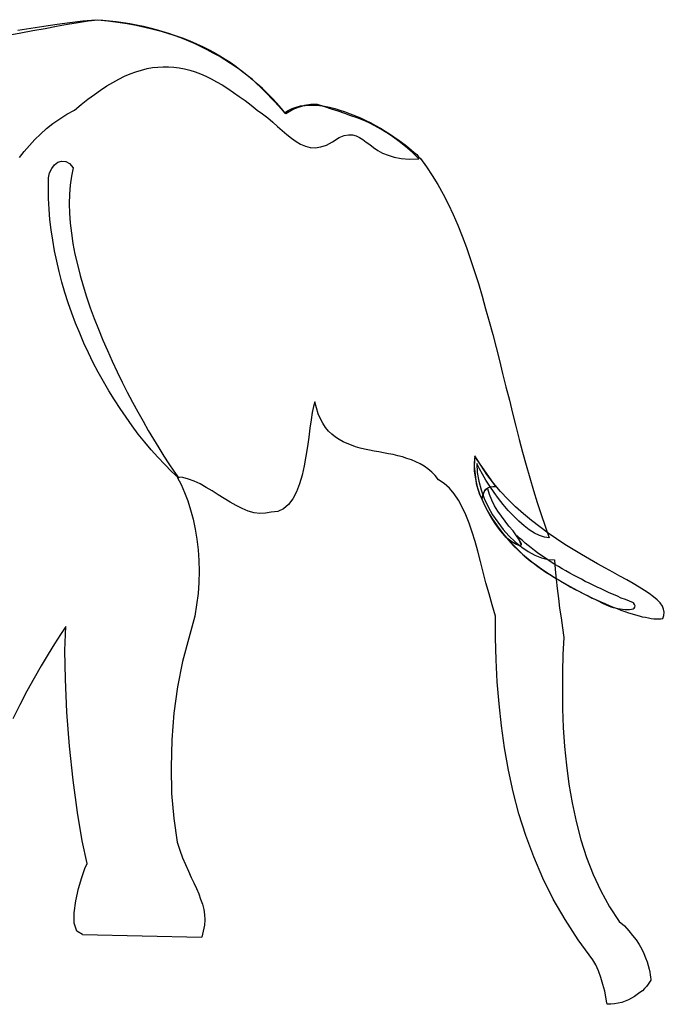
# Model space of a CAD drawing. Units: inches. Extents: x 386 to 107067, y -7 to 96314.
# Tile 10 of 10: x 107064.862 to 107066.855, y 96311.177 to 96314.222. Entities that reach past the tile are written whole.
import ezdxf

# ---------------------------------------------------------------- set-up
doc = ezdxf.new("R2010")
doc.units = ezdxf.units.IN
doc.layers.add('A-ELEV', color=7, linetype='Continuous', lineweight=25)
doc.layers.add('freecads.com', color=7, linetype='Continuous')

# ---------------------------------------------------------------- blocks, each defined once
blk = doc.blocks.new('elephant')
at = {"layer": 'freecads.com'}
for p, q in [((104458.6453, 95264.9047), (104458.6048, 95264.8987)), ((104458.6858, 95264.9107), (104458.6453, 95264.9047)), ((104458.6486, 95264.8987), (104458.6841, 95264.9052)), ((104458.6841, 95264.9052), (104458.7181, 95264.9113)), ((104458.7257, 95264.9162), (104458.6858, 95264.9107)), ((104458.7181, 95264.9113), (104458.7509, 95264.9167)), ((104458.7656, 95264.9206), (104458.7257, 95264.9162)), ((104458.7509, 95264.9167), (104458.782, 95264.9217)), ((104458.8055, 95264.9244), (104458.7656, 95264.9206)), ((104458.782, 95264.9217), (104458.8116, 95264.9255)), ((104458.8269, 95264.9227), (104458.8055, 95264.9244)), ((104458.8116, 95264.9255), (104458.8427, 95264.9222)), ((104458.8482, 95264.9211), (104458.8269, 95264.9227)), ((104458.8427, 95264.9222), (104458.8734, 95264.9178)), ((104458.869, 95264.9189), (104458.8482, 95264.9211)), ((104458.8903, 95264.9156), (104458.869, 95264.9189)), ((104458.8734, 95264.9178), (104458.9023, 95264.9134)), ((104458.9111, 95264.9124), (104458.8903, 95264.9156)), ((104458.9023, 95264.9134), (104458.9302, 95264.9085)), ((104458.9319, 95264.9085), (104458.9111, 95264.9124)), ((104458.9302, 95264.9085), (104458.957, 95264.9025)), ((104458.9527, 95264.9041), (104458.9319, 95264.9085)), ((104458.9734, 95264.8992), (104458.9527, 95264.9041)), ((104458.957, 95264.9025), (104458.9827, 95264.8965)), ((104458.5348, 95264.8773), (104458.5737, 95264.885)), ((104458.6048, 95264.8987), (104458.5644, 95264.8921)), ((104458.5737, 95264.885), (104458.6114, 95264.8921)), ((104458.6114, 95264.8921), (104458.6486, 95264.8987)), ((104458.9937, 95264.8938), (104458.9734, 95264.8992)), ((104458.9827, 95264.8965), (104459.0073, 95264.8899)), ((104459.0139, 95264.8877), (104458.9937, 95264.8938)), ((104459.0073, 95264.8899), (104459.0308, 95264.8828)), ((104459.0341, 95264.8812), (104459.0139, 95264.8877)), ((104459.0308, 95264.8828), (104459.0538, 95264.8757)), ((104459.0538, 95264.8741), (104459.0341, 95264.8812)), ((104459.0538, 95264.8757), (104459.0757, 95264.8681)), ((104459.0735, 95264.867), (104459.0538, 95264.8741)), ((104459.0932, 95264.8588), (104459.0735, 95264.867)), ((104459.0757, 95264.8681), (104459.0965, 95264.8599)), ((104459.1123, 95264.8506), (104459.0932, 95264.8588)), ((104459.0965, 95264.8599), (104459.1167, 95264.8511)), ((104459.1315, 95264.8418), (104459.1123, 95264.8506)), ((104459.1167, 95264.8511), (104459.1359, 95264.8424)), ((104459.1501, 95264.832), (104459.1315, 95264.8418)), ((104459.1359, 95264.8424), (104459.1544, 95264.8331)), ((104459.1687, 95264.8221), (104459.1501, 95264.832)), ((104459.1544, 95264.8331), (104459.1719, 95264.8238)), ((104459.1867, 95264.8123), (104459.1687, 95264.8221)), ((104459.1719, 95264.8238), (104459.1889, 95264.8139)), ((104459.2048, 95264.8013), (104459.1867, 95264.8123)), ((104459.1889, 95264.8139), (104459.2053, 95264.8035)), ((104458.9811, 95264.7773), (104458.9975, 95264.7789)), ((104458.9975, 95264.7789), (104459.0139, 95264.78)), ((104459.0139, 95264.78), (104459.0303, 95264.78)), ((104459.0303, 95264.78), (104459.0467, 95264.7789)), ((104459.0467, 95264.7789), (104459.0631, 95264.7767)), ((104459.2223, 95264.7899), (104459.2048, 95264.8013)), ((104459.2053, 95264.8035), (104459.2212, 95264.7937)), ((104459.2212, 95264.7937), (104459.2359, 95264.7833)), ((104459.2398, 95264.7784), (104459.2223, 95264.7899)), ((104459.2359, 95264.7833), (104459.2502, 95264.7724)), ((104458.8766, 95264.7412), (104458.8947, 95264.7505)), ((104458.8947, 95264.7505), (104458.9122, 95264.7581)), ((104458.9122, 95264.7581), (104458.9297, 95264.7642)), ((104458.9297, 95264.7642), (104458.9472, 95264.7696)), ((104458.9472, 95264.7696), (104458.9641, 95264.774)), ((104458.9641, 95264.774), (104458.9811, 95264.7773)), ((104459.0631, 95264.7767), (104459.0795, 95264.7735)), ((104459.0795, 95264.7735), (104459.0959, 95264.7691)), ((104459.0959, 95264.7691), (104459.1123, 95264.7642)), ((104459.1123, 95264.7642), (104459.1288, 95264.7576)), ((104459.1288, 95264.7576), (104459.1457, 95264.7505)), ((104459.1457, 95264.7505), (104459.1621, 95264.7423)), ((104459.2567, 95264.7658), (104459.2398, 95264.7784)), ((104459.2502, 95264.7724), (104459.2644, 95264.7614)), ((104459.2737, 95264.7532), (104459.2567, 95264.7658)), ((104459.2644, 95264.7614), (104459.2775, 95264.7505)), ((104459.2901, 95264.7401), (104459.2737, 95264.7532)), ((104459.2775, 95264.7505), (104459.2906, 95264.7395)), ((104458.8203, 95264.7078), (104458.8395, 95264.7204)), ((104458.8395, 95264.7204), (104458.8581, 95264.7313)), ((104458.8581, 95264.7313), (104458.8766, 95264.7412)), ((104459.1621, 95264.7423), (104459.179, 95264.7335)), ((104459.179, 95264.7335), (104459.196, 95264.7237)), ((104459.196, 95264.7237), (104459.2135, 95264.7128)), ((104459.3059, 95264.7264), (104459.2901, 95264.7401)), ((104459.2906, 95264.7395), (104459.3026, 95264.7281)), ((104459.3026, 95264.7281), (104459.3147, 95264.7171)), ((104459.3212, 95264.7122), (104459.3059, 95264.7264)), ((104458.7809, 95264.6794), (104458.8012, 95264.6942)), ((104458.8012, 95264.6942), (104458.8203, 95264.7078)), ((104459.2135, 95264.7128), (104459.231, 95264.7007)), ((104459.231, 95264.7007), (104459.2491, 95264.6882)), ((104459.2491, 95264.6882), (104459.2671, 95264.675)), ((104459.3147, 95264.7171), (104459.3262, 95264.7056)), ((104459.3366, 95264.6974), (104459.3212, 95264.7122)), ((104459.3262, 95264.7056), (104459.3376, 95264.6942)), ((104459.3513, 95264.6827), (104459.3366, 95264.6974)), ((104459.3376, 95264.6942), (104459.348, 95264.6827)), ((104458.7399, 95264.6455), (104458.7607, 95264.663)), ((104458.7607, 95264.663), (104458.7809, 95264.6794)), ((104459.2671, 95264.675), (104459.2857, 95264.6608)), ((104459.2857, 95264.6608), (104459.3043, 95264.6455)), ((104459.348, 95264.6827), (104459.359, 95264.6712)), ((104459.3655, 95264.6668), (104459.3513, 95264.6827)), ((104459.359, 95264.6712), (104459.3694, 95264.6597)), ((104459.3792, 95264.651), (104459.3655, 95264.6668)), ((104459.3694, 95264.6597), (104459.3792, 95264.6488)), ((104459.4251, 95264.6553), (104459.4383, 95264.6586)), ((104459.4383, 95264.6586), (104459.4525, 95264.6603)), ((104459.4443, 95264.6581), (104459.4383, 95264.6564)), ((104459.4508, 95264.6597), (104459.4443, 95264.6581)), ((104459.4574, 95264.6613), (104459.4508, 95264.6597)), ((104459.4525, 95264.6603), (104459.4667, 95264.6613)), ((104459.464, 95264.6624), (104459.4574, 95264.6613)), ((104459.4705, 95264.663), (104459.464, 95264.6624)), ((104459.4667, 95264.6613), (104459.4815, 95264.6613)), ((104459.4771, 95264.6635), (104459.4705, 95264.663)), ((104459.4842, 95264.6635), (104459.4771, 95264.6635)), ((104459.4815, 95264.6613), (104459.4968, 95264.6603)), ((104459.4908, 95264.663), (104459.4842, 95264.6635)), ((104459.5132, 95264.6559), (104459.4908, 95264.663)), ((104459.4968, 95264.6603), (104459.5127, 95264.6581)), ((104459.5127, 95264.6581), (104459.528, 95264.6548)), ((104458.6945, 95264.6192), (104458.7164, 95264.6329)), ((104458.7164, 95264.6329), (104458.7399, 95264.6455)), ((104459.3043, 95264.6455), (104459.3212, 95264.634)), ((104459.3212, 95264.634), (104459.3371, 95264.6214)), ((104459.3929, 95264.6345), (104459.3792, 95264.651)), ((104459.3792, 95264.6488), (104459.3891, 95264.6373)), ((104459.3891, 95264.6373), (104459.4005, 95264.6444)), ((104459.3978, 95264.6378), (104459.3929, 95264.6345)), ((104459.4033, 95264.6406), (104459.3978, 95264.6378)), ((104459.4005, 95264.6444), (104459.4126, 95264.6504)), ((104459.4087, 95264.6433), (104459.4033, 95264.6406)), ((104459.4142, 95264.6466), (104459.4087, 95264.6433)), ((104459.4126, 95264.6504), (104459.4251, 95264.6553)), ((104459.4197, 95264.6493), (104459.4142, 95264.6466)), ((104459.4257, 95264.6515), (104459.4197, 95264.6493)), ((104459.4317, 95264.6542), (104459.4257, 95264.6515)), ((104459.4383, 95264.6564), (104459.4317, 95264.6542)), ((104459.5345, 95264.6488), (104459.5132, 95264.6559)), ((104459.528, 95264.6548), (104459.5444, 95264.651)), ((104459.5553, 95264.6422), (104459.5345, 95264.6488)), ((104459.5444, 95264.651), (104459.5602, 95264.646)), ((104459.575, 95264.6356), (104459.5553, 95264.6422)), ((104459.5602, 95264.646), (104459.5761, 95264.6406)), ((104459.5941, 95264.6285), (104459.575, 95264.6356)), ((104459.5761, 95264.6406), (104459.5925, 95264.6345)), ((104459.5925, 95264.6345), (104459.6083, 95264.6285)), ((104459.6133, 95264.622), (104459.5941, 95264.6285)), ((104459.6083, 95264.6285), (104459.6242, 95264.6214)), ((104458.6535, 95264.5886), (104458.6732, 95264.6045)), ((104458.6732, 95264.6045), (104458.6945, 95264.6192)), ((104459.3371, 95264.6214), (104459.353, 95264.6083)), ((104459.353, 95264.6083), (104459.3677, 95264.5952)), ((104459.6319, 95264.6143), (104459.6133, 95264.622)), ((104459.6242, 95264.6214), (104459.6401, 95264.6138)), ((104459.6505, 95264.6061), (104459.6319, 95264.6143)), ((104459.6401, 95264.6138), (104459.6554, 95264.6061)), ((104459.6685, 95264.5974), (104459.6505, 95264.6061)), ((104459.6554, 95264.6061), (104459.6707, 95264.5979)), ((104459.6865, 95264.587), (104459.6685, 95264.5974)), ((104459.6707, 95264.5979), (104459.6855, 95264.5897)), ((104458.6174, 95264.5547), (104458.6349, 95264.5717)), ((104458.6349, 95264.5717), (104458.6535, 95264.5886)), ((104459.3677, 95264.5952), (104459.382, 95264.5826)), ((104459.382, 95264.5826), (104459.3962, 95264.57)), ((104459.3962, 95264.57), (104459.4104, 95264.5585)), ((104459.5575, 95264.5613), (104459.5733, 95264.5673)), ((104459.5733, 95264.5673), (104459.587, 95264.5695)), ((104459.587, 95264.5695), (104459.5996, 95264.5689)), ((104459.5996, 95264.5689), (104459.6105, 95264.5662)), ((104459.6105, 95264.5662), (104459.6209, 95264.5613)), ((104459.6855, 95264.5897), (104459.6997, 95264.581)), ((104459.7051, 95264.576), (104459.6865, 95264.587)), ((104459.6997, 95264.581), (104459.7133, 95264.5722)), ((104459.7243, 95264.5629), (104459.7051, 95264.576)), ((104459.7133, 95264.5722), (104459.7265, 95264.5635)), ((104458.5846, 95264.5181), (104458.6005, 95264.5367)), ((104458.6005, 95264.5367), (104458.6174, 95264.5547)), ((104459.4104, 95264.5585), (104459.4246, 95264.5487)), ((104459.4246, 95264.5487), (104459.4388, 95264.5405)), ((104459.4388, 95264.5405), (104459.4536, 95264.5345)), ((104459.5012, 95264.5317), (104459.5187, 95264.5378)), ((104459.5187, 95264.5378), (104459.5373, 95264.5476)), ((104459.5373, 95264.5476), (104459.5575, 95264.5613)), ((104459.6209, 95264.5613), (104459.6313, 95264.5547)), ((104459.6313, 95264.5547), (104459.6417, 95264.5471)), ((104459.6417, 95264.5471), (104459.6526, 95264.5389)), ((104459.6526, 95264.5389), (104459.6641, 95264.5301)), ((104459.7434, 95264.5487), (104459.7243, 95264.5629)), ((104459.7265, 95264.5635), (104459.739, 95264.5553)), ((104459.739, 95264.5553), (104459.7511, 95264.5465)), ((104459.7631, 95264.5328), (104459.7434, 95264.5487)), ((104459.7511, 95264.5465), (104459.762, 95264.5383)), ((104459.762, 95264.5383), (104459.7724, 95264.5301)), ((104458.5693, 95264.4995), (104458.5846, 95264.5181)), ((104459.4536, 95264.5345), (104459.4683, 95264.5306)), ((104459.4683, 95264.5306), (104459.4842, 95264.5296)), ((104459.4842, 95264.5296), (104459.5012, 95264.5317)), ((104459.6641, 95264.5301), (104459.6773, 95264.5213)), ((104459.6773, 95264.5213), (104459.692, 95264.5131)), ((104459.692, 95264.5131), (104459.709, 95264.506)), ((104459.709, 95264.506), (104459.7281, 95264.5)), ((104459.7833, 95264.5153), (104459.7631, 95264.5328)), ((104459.7724, 95264.5301), (104459.7817, 95264.5224)), ((104459.7817, 95264.5224), (104459.7899, 95264.5148)), ((104459.8047, 95264.4951), (104459.7833, 95264.5153)), ((104459.7899, 95264.5148), (104459.7976, 95264.5082)), ((104459.7976, 95264.5082), (104459.8036, 95264.5017)), ((104458.6694, 95264.4656), (104458.6781, 95264.4765)), ((104458.6781, 95264.4765), (104458.6885, 95264.4847)), ((104458.6885, 95264.4847), (104458.7, 95264.488)), ((104458.7, 95264.488), (104458.7126, 95264.4869)), ((104458.7126, 95264.4869), (104458.7246, 95264.4803)), ((104458.7246, 95264.4803), (104458.7361, 95264.4672)), ((104459.7281, 95264.5), (104459.75, 95264.4962)), ((104459.75, 95264.4962), (104459.7757, 95264.4945)), ((104459.7757, 95264.4945), (104459.8047, 95264.4951)), ((104459.8036, 95264.5017), (104459.809, 95264.4956)), ((104459.809, 95264.4956), (104459.8276, 95264.4705)), ((104458.6595, 95264.436), (104458.6628, 95264.4519)), ((104458.6628, 95264.4519), (104458.6694, 95264.4656)), ((104458.7361, 95264.4672), (104458.7301, 95264.441)), ((104459.8276, 95264.4705), (104459.8457, 95264.4437)), ((104459.8457, 95264.4437), (104459.8632, 95264.4158)), ((104458.659, 95264.4043), (104458.6595, 95264.436)), ((104458.7263, 95264.4136), (104458.7241, 95264.3857)), ((104458.7301, 95264.441), (104458.7263, 95264.4136)), ((104459.8632, 95264.4158), (104459.8796, 95264.3863)), ((104458.6595, 95264.3721), (104458.659, 95264.4043)), ((104458.7241, 95264.3857), (104458.723, 95264.3562)), ((104459.8796, 95264.3863), (104459.8949, 95264.3556)), ((104458.6612, 95264.3398), (104458.6595, 95264.3721)), ((104458.723, 95264.3562), (104458.7241, 95264.3267)), ((104459.8949, 95264.3556), (104459.9102, 95264.3234)), ((104458.6639, 95264.3075), (104458.6612, 95264.3398)), ((104458.7241, 95264.3267), (104458.7263, 95264.296)), ((104459.9102, 95264.3234), (104459.9244, 95264.29)), ((104458.6677, 95264.2753), (104458.6639, 95264.3075)), ((104458.7263, 95264.296), (104458.7301, 95264.2649)), ((104458.6727, 95264.243), (104458.6677, 95264.2753)), ((104458.7301, 95264.2649), (104458.735, 95264.2331)), ((104459.9244, 95264.29), (104459.9381, 95264.2556)), ((104458.6781, 95264.2107), (104458.6727, 95264.243)), ((104458.735, 95264.2331), (104458.741, 95264.2003)), ((104459.9381, 95264.2556), (104459.9512, 95264.2206)), ((104458.6847, 95264.1785), (104458.6781, 95264.2107)), ((104458.741, 95264.2003), (104458.7487, 95264.1681)), ((104459.9512, 95264.2206), (104459.9643, 95264.1839)), ((104458.6924, 95264.1462), (104458.6847, 95264.1785)), ((104459.9643, 95264.1839), (104459.9764, 95264.1468)), ((104458.7011, 95264.1139), (104458.6924, 95264.1462)), ((104458.7487, 95264.1681), (104458.7569, 95264.1347)), ((104459.9764, 95264.1468), (104459.9884, 95264.109)), ((104458.7104, 95264.0817), (104458.7011, 95264.1139)), ((104458.7569, 95264.1347), (104458.7667, 95264.1019)), ((104459.9884, 95264.109), (104459.9999, 95264.0707)), ((104458.7202, 95264.0499), (104458.7104, 95264.0817)), ((104458.7667, 95264.1019), (104458.7771, 95264.0685)), ((104458.7312, 95264.0182), (104458.7202, 95264.0499)), ((104458.7771, 95264.0685), (104458.7886, 95264.0346)), ((104459.9999, 95264.0707), (104460.0108, 95264.0314)), ((104458.7432, 95263.9871), (104458.7312, 95264.0182)), ((104458.7886, 95264.0346), (104458.8006, 95264.0013)), ((104460.0108, 95264.0314), (104460.0218, 95263.992)), ((104458.7558, 95263.9559), (104458.7432, 95263.9871)), ((104458.8006, 95264.0013), (104458.8138, 95263.9679)), ((104460.0218, 95263.992), (104460.0327, 95263.9521)), ((104458.8138, 95263.9679), (104458.8274, 95263.9346)), ((104458.7689, 95263.9253), (104458.7558, 95263.9559)), ((104458.8274, 95263.9346), (104458.8416, 95263.9018)), ((104460.0327, 95263.9521), (104460.0431, 95263.9116)), ((104458.7831, 95263.8946), (104458.7689, 95263.9253)), ((104458.8416, 95263.9018), (104458.8559, 95263.8689)), ((104460.0431, 95263.9116), (104460.0535, 95263.8711)), ((104458.7973, 95263.8646), (104458.7831, 95263.8946)), ((104458.8559, 95263.8689), (104458.8712, 95263.8367)), ((104460.0535, 95263.8711), (104460.0633, 95263.8307)), ((104458.8132, 95263.835), (104458.7973, 95263.8646)), ((104458.8291, 95263.806), (104458.8132, 95263.835)), ((104458.8712, 95263.8367), (104458.887, 95263.8044)), ((104458.8455, 95263.7776), (104458.8291, 95263.806)), ((104458.887, 95263.8044), (104458.9029, 95263.7732)), ((104460.0633, 95263.8307), (104460.0737, 95263.7896)), ((104458.863, 95263.7497), (104458.8455, 95263.7776)), ((104460.0737, 95263.7896), (104460.0841, 95263.7486)), ((104458.8805, 95263.7224), (104458.863, 95263.7497)), ((104458.9029, 95263.7732), (104458.9187, 95263.7426)), ((104459.4831, 95263.7437), (104459.4787, 95263.7289)), ((104459.4875, 95263.7246), (104459.4831, 95263.7437)), ((104460.0841, 95263.7486), (104460.094, 95263.7082)), ((104458.8991, 95263.6956), (104458.8805, 95263.7224)), ((104458.9187, 95263.7426), (104458.9352, 95263.7125)), ((104459.4787, 95263.7289), (104459.4749, 95263.7103)), ((104459.4935, 95263.7065), (104459.4875, 95263.7246)), ((104458.9176, 95263.6694), (104458.8991, 95263.6956)), ((104458.9352, 95263.7125), (104458.9516, 95263.6835)), ((104458.9516, 95263.6835), (104458.968, 95263.6551)), ((104459.4711, 95263.6874), (104459.4678, 95263.6622)), ((104459.4749, 95263.7103), (104459.4711, 95263.6874)), ((104459.5001, 95263.6912), (104459.4935, 95263.7065)), ((104459.5077, 95263.677), (104459.5001, 95263.6912)), ((104460.094, 95263.7082), (104460.1043, 95263.6677)), ((104458.9368, 95263.6436), (104458.9176, 95263.6694)), ((104458.968, 95263.6551), (104458.9838, 95263.6278)), ((104459.4678, 95263.6622), (104459.464, 95263.6343)), ((104459.5159, 95263.6639), (104459.5077, 95263.677)), ((104459.5252, 95263.6529), (104459.5159, 95263.6639)), ((104459.5356, 95263.6431), (104459.5252, 95263.6529)), ((104460.1043, 95263.6677), (104460.1147, 95263.6272)), ((104458.957, 95263.619), (104458.9368, 95263.6436)), ((104458.9838, 95263.6278), (104459.0002, 95263.601)), ((104459.464, 95263.6343), (104459.4601, 95263.6054)), ((104459.5466, 95263.6343), (104459.5356, 95263.6431)), ((104459.558, 95263.6267), (104459.5466, 95263.6343)), ((104459.5701, 95263.6196), (104459.558, 95263.6267)), ((104460.1147, 95263.6272), (104460.1251, 95263.5873)), ((104458.9773, 95263.595), (104458.957, 95263.619)), ((104458.9975, 95263.572), (104458.9773, 95263.595)), ((104459.0002, 95263.601), (104459.0161, 95263.5758)), ((104459.4601, 95263.6054), (104459.4552, 95263.5753)), ((104459.5826, 95263.6141), (104459.5701, 95263.6196)), ((104459.5958, 95263.6092), (104459.5826, 95263.6141)), ((104459.6089, 95263.6043), (104459.5958, 95263.6092)), ((104459.6226, 95263.6004), (104459.6089, 95263.6043)), ((104459.6368, 95263.5972), (104459.6226, 95263.6004)), ((104459.6516, 95263.5944), (104459.6368, 95263.5972)), ((104459.6658, 95263.5912), (104459.6516, 95263.5944)), ((104459.6805, 95263.5884), (104459.6658, 95263.5912)), ((104459.0188, 95263.5496), (104458.9975, 95263.572)), ((104459.0161, 95263.5758), (104459.0319, 95263.5518)), ((104459.4552, 95263.5753), (104459.4497, 95263.5458)), ((104459.6953, 95263.5857), (104459.6805, 95263.5884)), ((104459.7101, 95263.583), (104459.6953, 95263.5857)), ((104459.7248, 95263.5802), (104459.7101, 95263.583)), ((104459.739, 95263.5769), (104459.7248, 95263.5802)), ((104459.7533, 95263.5731), (104459.739, 95263.5769)), ((104459.7675, 95263.5687), (104459.7533, 95263.5731)), ((104459.7817, 95263.5638), (104459.7675, 95263.5687)), ((104459.7948, 95263.5583), (104459.7817, 95263.5638)), ((104459.9775, 95263.5769), (104459.9753, 95263.5534)), ((104459.9764, 95263.5605), (104459.9758, 95263.5447)), ((104459.9775, 95263.5748), (104459.9764, 95263.5605)), ((104459.9955, 95263.5474), (104459.9775, 95263.5769)), ((104460.042, 95263.4812), (104459.9775, 95263.5748)), ((104460.1251, 95263.5873), (104460.1361, 95263.5474)), ((104459.0401, 95263.5283), (104459.0188, 95263.5496)), ((104459.0319, 95263.5518), (104459.0473, 95263.5288)), ((104459.4497, 95263.5458), (104459.4432, 95263.5168)), ((104459.808, 95263.5518), (104459.7948, 95263.5583)), ((104459.8205, 95263.5441), (104459.808, 95263.5518)), ((104459.8326, 95263.5359), (104459.8205, 95263.5441)), ((104459.8446, 95263.5261), (104459.8326, 95263.5359)), ((104459.9753, 95263.5534), (104459.9758, 95263.5294)), ((104459.9758, 95263.5447), (104459.9769, 95263.5272)), ((104459.9917, 95263.5365), (104459.9835, 95263.5523)), ((104459.9835, 95263.5523), (104459.9851, 95263.525)), ((104460.001, 95263.5195), (104459.9917, 95263.5365)), ((104460.0147, 95263.519), (104459.9955, 95263.5474)), ((104460.1361, 95263.5474), (104460.147, 95263.5086)), ((104459.062, 95263.5075), (104459.0401, 95263.5283)), ((104459.0473, 95263.5288), (104459.062, 95263.5075)), ((104459.0746, 95263.5091), (104459.0576, 95263.5108)), ((104459.0576, 95263.5108), (104459.0691, 95263.4878)), ((104459.0921, 95263.5047), (104459.0746, 95263.5091)), ((104459.1102, 95263.4982), (104459.0921, 95263.5047)), ((104459.4432, 95263.5168), (104459.4355, 95263.49)), ((104459.855, 95263.5151), (104459.8446, 95263.5261)), ((104459.8654, 95263.5026), (104459.855, 95263.5151)), ((104459.8829, 95263.4911), (104459.8654, 95263.5026)), ((104459.9758, 95263.5294), (104459.9791, 95263.5053)), ((104459.9769, 95263.5272), (104459.9791, 95263.5091)), ((104459.9791, 95263.5091), (104459.9818, 95263.4911)), ((104459.9791, 95263.5053), (104459.9851, 95263.4807)), ((104459.9851, 95263.525), (104459.9895, 95263.4976)), ((104460.0119, 95263.5009), (104460.001, 95263.5195)), ((104460.024, 95263.4823), (104460.0119, 95263.5009)), ((104460.0349, 95263.4922), (104460.0147, 95263.519)), ((104460.147, 95263.5086), (104460.1585, 95263.4697)), ((104459.0691, 95263.4878), (104459.0801, 95263.4632)), ((104459.1282, 95263.4894), (104459.1102, 95263.4982)), ((104459.1468, 95263.479), (104459.1282, 95263.4894)), ((104459.1654, 95263.4681), (104459.1468, 95263.479)), ((104459.4355, 95263.49), (104459.4257, 95263.4648)), ((104459.8987, 95263.4763), (104459.8829, 95263.4911)), ((104459.9135, 95263.4594), (104459.8987, 95263.4763)), ((104459.9818, 95263.4911), (104459.9868, 95263.4736)), ((104459.9851, 95263.4807), (104459.9933, 95263.4561)), ((104459.9868, 95263.4736), (104459.9922, 95263.4572)), ((104459.9895, 95263.4976), (104459.9966, 95263.4708)), ((104459.9966, 95263.4708), (104460.0065, 95263.4446)), ((104460.007, 95263.4676), (104460.0119, 95263.4736)), ((104460.0103, 95263.4703), (104460.0076, 95263.467)), ((104460.0136, 95263.473), (104460.0103, 95263.4703)), ((104460.0119, 95263.4736), (104460.0179, 95263.4774)), ((104460.0174, 95263.4747), (104460.0136, 95263.473)), ((104460.0229, 95263.4566), (104460.0174, 95263.4747)), ((104460.0179, 95263.4774), (104460.0245, 95263.4801)), ((104460.0371, 95263.4632), (104460.024, 95263.4823)), ((104460.0245, 95263.4801), (104460.0327, 95263.4812)), ((104460.0327, 95263.4812), (104460.042, 95263.4812)), ((104460.0568, 95263.4665), (104460.0349, 95263.4922)), ((104460.1585, 95263.4697), (104460.17, 95263.432)), ((104459.0801, 95263.4632), (104459.0899, 95263.4369)), ((104459.184, 95263.4561), (104459.1654, 95263.4681)), ((104459.2026, 95263.4446), (104459.184, 95263.4561)), ((104459.2212, 95263.4331), (104459.2026, 95263.4446)), ((104459.4148, 95263.4435), (104459.4016, 95263.4255)), ((104459.4257, 95263.4648), (104459.4148, 95263.4435)), ((104459.9266, 95263.4397), (104459.9135, 95263.4594)), ((104459.9387, 95263.4178), (104459.9266, 95263.4397)), ((104459.9922, 95263.4572), (104459.9999, 95263.4424)), ((104459.9933, 95263.4561), (104460.0037, 95263.4315)), ((104460.0004, 95263.4473), (104459.9988, 95263.4419)), ((104459.9988, 95263.4419), (104460.0065, 95263.4255)), ((104459.9999, 95263.4424), (104460.001, 95263.4522)), ((104460.0021, 95263.4528), (104460.0004, 95263.4473)), ((104460.001, 95263.4522), (104460.0037, 95263.461)), ((104460.0032, 95263.4577), (104460.0021, 95263.4528)), ((104460.0054, 95263.4626), (104460.0032, 95263.4577)), ((104460.0037, 95263.461), (104460.007, 95263.4676)), ((104460.0076, 95263.467), (104460.0054, 95263.4626)), ((104460.0065, 95263.4446), (104460.0185, 95263.4189)), ((104460.03, 95263.4397), (104460.0229, 95263.4566)), ((104460.0387, 95263.4222), (104460.03, 95263.4397)), ((104460.0508, 95263.444), (104460.0371, 95263.4632)), ((104460.0655, 95263.4255), (104460.0508, 95263.444)), ((104460.0797, 95263.4424), (104460.0568, 95263.4665)), ((104460.1033, 95263.4189), (104460.0797, 95263.4424)), ((104459.0899, 95263.4369), (104459.0987, 95263.4091)), ((104459.0987, 95263.4091), (104459.1063, 95263.3801)), ((104459.2398, 95263.4227), (104459.2212, 95263.4331)), ((104459.2584, 95263.4134), (104459.2398, 95263.4227)), ((104459.2769, 95263.4058), (104459.2584, 95263.4134)), ((104459.3858, 95263.4123), (104459.3683, 95263.4041)), ((104459.4016, 95263.4255), (104459.3858, 95263.4123)), ((104459.9496, 95263.3937), (104459.9387, 95263.4178)), ((104460.0037, 95263.4315), (104460.0158, 95263.4074)), ((104460.0065, 95263.4255), (104460.0141, 95263.4101)), ((104460.0141, 95263.4101), (104460.0212, 95263.3965)), ((104460.0185, 95263.4189), (104460.0322, 95263.3943)), ((104460.0486, 95263.4058), (104460.0387, 95263.4222)), ((104460.0808, 95263.4074), (104460.0655, 95263.4255)), ((104460.1279, 95263.397), (104460.1033, 95263.4189)), ((104460.17, 95263.432), (104460.182, 95263.3948)), ((104459.1063, 95263.3801), (104459.1129, 95263.3494)), ((104459.295, 95263.4003), (104459.2769, 95263.4058)), ((104459.313, 95263.3981), (104459.295, 95263.4003)), ((104459.3305, 95263.3987), (104459.313, 95263.3981)), ((104459.3475, 95263.4025), (104459.3305, 95263.3987)), ((104459.3683, 95263.4041), (104459.3475, 95263.4025)), ((104459.9594, 95263.368), (104459.9496, 95263.3937)), ((104460.0158, 95263.4074), (104460.03, 95263.3833)), ((104460.0212, 95263.3965), (104460.0289, 95263.3833)), ((104460.0289, 95263.3833), (104460.0371, 95263.3702)), ((104460.03, 95263.3833), (104460.0464, 95263.3598)), ((104460.0322, 95263.3943), (104460.048, 95263.3708)), ((104460.0595, 95263.3899), (104460.0486, 95263.4058)), ((104460.071, 95263.374), (104460.0595, 95263.3899)), ((104460.0967, 95263.3905), (104460.0808, 95263.4074)), ((104460.1131, 95263.3746), (104460.0967, 95263.3905)), ((104460.1525, 95263.3762), (104460.1279, 95263.397)), ((104460.182, 95263.3948), (104460.1946, 95263.3587)), ((104459.1129, 95263.3494), (104459.1178, 95263.3183)), ((104459.9687, 95263.3407), (104459.9594, 95263.368)), ((104460.0371, 95263.3702), (104460.0464, 95263.3571)), ((104460.0464, 95263.3598), (104460.0639, 95263.3363)), ((104460.0464, 95263.3571), (104460.0568, 95263.3434)), ((104460.048, 95263.3708), (104460.065, 95263.3489)), ((104460.065, 95263.3489), (104460.083, 95263.3287)), ((104460.083, 95263.3587), (104460.071, 95263.374)), ((104460.0956, 95263.344), (104460.083, 95263.3587)), ((104460.1295, 95263.3598), (104460.1131, 95263.3746)), ((104460.1454, 95263.3478), (104460.1295, 95263.3598)), ((104460.1618, 95263.3374), (104460.1454, 95263.3478)), ((104460.1782, 95263.3565), (104460.1525, 95263.3762)), ((104460.2039, 95263.3374), (104460.1782, 95263.3565)), ((104460.1946, 95263.3587), (104460.2077, 95263.3232)), ((104459.1178, 95263.3183), (104459.1216, 95263.286)), ((104459.978, 95263.3117), (104459.9687, 95263.3407)), ((104460.0568, 95263.3434), (104460.0688, 95263.3287)), ((104460.0639, 95263.3363), (104460.083, 95263.3144)), ((104460.0688, 95263.3287), (104460.0715, 95263.3265)), ((104460.0715, 95263.3265), (104460.0754, 95263.3237)), ((104460.0754, 95263.3237), (104460.0803, 95263.3199)), ((104460.0803, 95263.3199), (104460.0863, 95263.3155)), ((104460.083, 95263.3287), (104460.1022, 95263.3101)), ((104460.106, 95263.3292), (104460.0956, 95263.344)), ((104460.1136, 95263.3183), (104460.106, 95263.3292)), ((104460.1076, 95263.3297), (104460.1125, 95263.321)), ((104460.1158, 95263.3221), (104460.1076, 95263.3297)), ((104460.1125, 95263.321), (104460.1169, 95263.3128)), ((104460.118, 95263.3095), (104460.1136, 95263.3183)), ((104460.1246, 95263.3144), (104460.1158, 95263.3221)), ((104460.1776, 95263.3297), (104460.1618, 95263.3374)), ((104460.193, 95263.3248), (104460.1776, 95263.3297)), ((104460.2077, 95263.3232), (104460.193, 95263.3248)), ((104460.2301, 95263.3194), (104460.2039, 95263.3374)), ((104460.2558, 95263.3024), (104460.2301, 95263.3194)), ((104459.9862, 95263.2811), (104459.978, 95263.3117)), ((104460.1, 95263.3051), (104460.0814, 95263.3161)), ((104460.0814, 95263.3161), (104460.0961, 95263.2991)), ((104460.083, 95263.3144), (104460.1038, 95263.2926)), ((104460.0863, 95263.3155), (104460.0923, 95263.3112)), ((104460.0923, 95263.3112), (104460.0989, 95263.3073)), ((104460.0961, 95263.2991), (104460.1125, 95263.2833)), ((104460.0989, 95263.3073), (104460.1049, 95263.3035)), ((104460.112, 95263.2997), (104460.1, 95263.3051)), ((104460.1022, 95263.3101), (104460.1224, 95263.2942)), ((104460.1038, 95263.2926), (104460.1251, 95263.2718)), ((104460.1049, 95263.3035), (104460.1104, 95263.3008)), ((104460.1104, 95263.3008), (104460.1147, 95263.2991)), ((104460.1186, 95263.2986), (104460.112, 95263.2997)), ((104460.1147, 95263.2991), (104460.1186, 95263.2991)), ((104460.1169, 95263.3128), (104460.1202, 95263.3057)), ((104460.1202, 95263.3041), (104460.118, 95263.3095)), ((104460.1207, 95263.3008), (104460.1186, 95263.2986)), ((104460.1186, 95263.2991), (104460.1202, 95263.3002)), ((104460.1202, 95263.3057), (104460.1207, 95263.3008)), ((104460.1202, 95263.3002), (104460.1202, 95263.3041)), ((104460.1224, 95263.2942), (104460.1426, 95263.2805)), ((104460.1333, 95263.3068), (104460.1246, 95263.3144)), ((104460.1426, 95263.2991), (104460.1333, 95263.3068)), ((104460.1519, 95263.2915), (104460.1426, 95263.2991)), ((104460.1618, 95263.2838), (104460.1519, 95263.2915)), ((104460.2815, 95263.2866), (104460.2558, 95263.3024)), ((104460.3072, 95263.2712), (104460.2815, 95263.2866)), ((104459.1216, 95263.286), (104459.1238, 95263.2532)), ((104459.995, 95263.2499), (104459.9862, 95263.2811)), ((104460.1125, 95263.2833), (104460.13, 95263.2674)), ((104460.1251, 95263.2718), (104460.1481, 95263.2526)), ((104460.13, 95263.2674), (104460.1481, 95263.2521)), ((104460.1426, 95263.2805), (104460.1634, 95263.2696)), ((104460.1716, 95263.2767), (104460.1618, 95263.2838)), ((104460.1634, 95263.2696), (104460.1837, 95263.2614)), ((104460.1815, 95263.2691), (104460.1716, 95263.2767)), ((104460.1924, 95263.2619), (104460.1815, 95263.2691)), ((104460.1837, 95263.2614), (104460.2039, 95263.2559)), ((104460.2028, 95263.2548), (104460.1924, 95263.2619)), ((104460.2039, 95263.2559), (104460.2236, 95263.2543)), ((104460.3324, 95263.2565), (104460.3072, 95263.2712)), ((104460.357, 95263.2428), (104460.3324, 95263.2565)), ((104459.1238, 95263.2532), (104459.1249, 95263.2193)), ((104460.0032, 95263.2171), (104459.995, 95263.2499)), ((104460.1481, 95263.2526), (104460.1722, 95263.234)), ((104460.1481, 95263.2521), (104460.1678, 95263.2379)), ((104460.1678, 95263.2379), (104460.1875, 95263.2237)), ((104460.1722, 95263.234), (104460.1968, 95263.2171)), ((104460.2137, 95263.2477), (104460.2028, 95263.2548)), ((104460.2247, 95263.2406), (104460.2137, 95263.2477)), ((104460.2236, 95263.2543), (104460.2258, 95263.2247)), ((104460.2361, 95263.234), (104460.2247, 95263.2406)), ((104460.2476, 95263.2269), (104460.2361, 95263.234)), ((104460.2591, 95263.2204), (104460.2476, 95263.2269)), ((104460.3811, 95263.2291), (104460.357, 95263.2428)), ((104460.404, 95263.2165), (104460.3811, 95263.2291)), ((104459.1249, 95263.2193), (104459.1238, 95263.1848)), ((104460.0119, 95263.1837), (104460.0032, 95263.2171)), ((104460.1875, 95263.2237), (104460.2083, 95263.21)), ((104460.1968, 95263.2171), (104460.2094, 95263.2089)), ((104460.2083, 95263.21), (104460.229, 95263.1969)), ((104460.2094, 95263.2089), (104460.2219, 95263.2012)), ((104460.2219, 95263.2012), (104460.235, 95263.1936)), ((104460.2258, 95263.2247), (104460.229, 95263.1952)), ((104460.229, 95263.1969), (104460.2504, 95263.1843)), ((104460.229, 95263.1952), (104460.2323, 95263.1657)), ((104460.2706, 95263.2138), (104460.2591, 95263.2204)), ((104460.2826, 95263.2072), (104460.2706, 95263.2138)), ((104460.2947, 95263.2007), (104460.2826, 95263.2072)), ((104460.3067, 95263.1947), (104460.2947, 95263.2007)), ((104460.4259, 95263.2045), (104460.404, 95263.2165)), ((104460.4472, 95263.193), (104460.4259, 95263.2045)), ((104459.1238, 95263.1848), (104459.1216, 95263.1504)), ((104460.0212, 95263.1498), (104460.0119, 95263.1837)), ((104460.2323, 95263.1657), (104460.2356, 95263.1356)), ((104460.235, 95263.1936), (104460.2482, 95263.1854)), ((104460.2482, 95263.1854), (104460.2613, 95263.1783)), ((104460.2504, 95263.1843), (104460.2717, 95263.1723)), ((104460.2613, 95263.1783), (104460.2744, 95263.1706)), ((104460.2717, 95263.1723), (104460.293, 95263.1608)), ((104460.2744, 95263.1706), (104460.2875, 95263.1635)), ((104460.3187, 95263.1881), (104460.3067, 95263.1947)), ((104460.3313, 95263.1821), (104460.3187, 95263.1881)), ((104460.3433, 95263.1761), (104460.3313, 95263.1821)), ((104460.3559, 95263.1701), (104460.3433, 95263.1761)), ((104460.3679, 95263.1646), (104460.3559, 95263.1701)), ((104460.3805, 95263.1586), (104460.3679, 95263.1646)), ((104460.4669, 95263.1816), (104460.4472, 95263.193)), ((104460.485, 95263.1706), (104460.4669, 95263.1816)), ((104460.5019, 95263.1602), (104460.485, 95263.1706)), ((104459.1216, 95263.1504), (104459.1173, 95263.1159)), ((104460.0305, 95263.1154), (104460.0212, 95263.1498)), ((104460.2356, 95263.1356), (104460.2394, 95263.1055)), ((104460.2875, 95263.1635), (104460.3012, 95263.1564)), ((104460.293, 95263.1608), (104460.3144, 95263.1498)), ((104460.3012, 95263.1564), (104460.3144, 95263.1498)), ((104460.3144, 95263.1498), (104460.3346, 95263.1394)), ((104460.3144, 95263.1498), (104460.3275, 95263.1433)), ((104460.3275, 95263.1433), (104460.3406, 95263.1367)), ((104460.3346, 95263.1394), (104460.3548, 95263.1296)), ((104460.3406, 95263.1367), (104460.3537, 95263.1307)), ((104460.3931, 95263.1531), (104460.3805, 95263.1586)), ((104460.4057, 95263.1477), (104460.3931, 95263.1531)), ((104460.4182, 95263.1422), (104460.4057, 95263.1477)), ((104460.4303, 95263.1367), (104460.4182, 95263.1422)), ((104460.4429, 95263.1318), (104460.4303, 95263.1367)), ((104460.5167, 95263.1504), (104460.5019, 95263.1602)), ((104460.5298, 95263.1405), (104460.5167, 95263.1504)), ((104460.5413, 95263.1307), (104460.5298, 95263.1405)), ((104459.1173, 95263.1159), (104459.1113, 95263.0809)), ((104460.0409, 95263.0804), (104460.0305, 95263.1154)), ((104460.2394, 95263.1055), (104460.2438, 95263.0749)), ((104460.3537, 95263.1307), (104460.3668, 95263.1247)), ((104460.3548, 95263.1296), (104460.3745, 95263.1198)), ((104460.3668, 95263.1247), (104460.3794, 95263.1192)), ((104460.3745, 95263.1198), (104460.3931, 95263.111)), ((104460.3794, 95263.1192), (104460.3925, 95263.1137)), ((104460.3925, 95263.1137), (104460.4046, 95263.1088)), ((104460.3931, 95263.111), (104460.398, 95263.1094)), ((104460.398, 95263.1094), (104460.4046, 95263.1077)), ((104460.4046, 95263.1088), (104460.4172, 95263.1039)), ((104460.4046, 95263.1077), (104460.4111, 95263.1061)), ((104460.4111, 95263.1061), (104460.4188, 95263.1044)), ((104460.4172, 95263.1039), (104460.4292, 95263.099)), ((104460.4188, 95263.1044), (104460.4265, 95263.1028)), ((104460.4554, 95263.1269), (104460.4429, 95263.1318)), ((104460.4675, 95263.1219), (104460.4554, 95263.1269)), ((104460.4669, 95263.1033), (104460.4702, 95263.1055)), ((104460.4713, 95263.1165), (104460.4675, 95263.1219)), ((104460.4702, 95263.1055), (104460.4724, 95263.1083)), ((104460.4729, 95263.1121), (104460.4713, 95263.1165)), ((104460.4724, 95263.1083), (104460.4729, 95263.1121)), ((104460.55, 95263.1214), (104460.5413, 95263.1307)), ((104460.5572, 95263.1116), (104460.55, 95263.1214)), ((104460.561, 95263.1023), (104460.5572, 95263.1116)), ((104459.1113, 95263.0809), (104459.103, 95263.0465)), ((104460.0415, 95263.0131), (104460.0409, 95263.0804)), ((104460.2438, 95263.0749), (104460.2482, 95263.0448)), ((104460.4265, 95263.1028), (104460.4341, 95263.1023)), ((104460.4292, 95263.099), (104460.4407, 95263.0951)), ((104460.4341, 95263.1023), (104460.4423, 95263.1012)), ((104460.4407, 95263.0951), (104460.4522, 95263.0913)), ((104460.4423, 95263.1012), (104460.4494, 95263.1012)), ((104460.4494, 95263.1012), (104460.456, 95263.1012)), ((104460.4522, 95263.0913), (104460.4637, 95263.0875)), ((104460.456, 95263.1012), (104460.462, 95263.1023)), ((104460.462, 95263.1023), (104460.4669, 95263.1033)), ((104460.4637, 95263.0875), (104460.4746, 95263.0842)), ((104460.4746, 95263.0842), (104460.485, 95263.0815)), ((104460.485, 95263.0815), (104460.4948, 95263.0787)), ((104460.4948, 95263.0787), (104460.5047, 95263.0771)), ((104460.5047, 95263.0771), (104460.5139, 95263.0749)), ((104460.5139, 95263.0749), (104460.5227, 95263.0738)), ((104460.5227, 95263.0738), (104460.5309, 95263.0727)), ((104460.5522, 95263.0727), (104460.5582, 95263.0738)), ((104460.5582, 95263.0738), (104460.5621, 95263.0831)), ((104460.5632, 95263.093), (104460.561, 95263.1023)), ((104460.5621, 95263.0831), (104460.5632, 95263.093)), ((104458.7131, 95263.0481), (104458.6967, 95263.0241)), ((104458.7099, 95262.9748), (104458.7131, 95263.0481)), ((104459.103, 95263.0465), (104459.0932, 95263.012)), ((104460.2482, 95263.0448), (104460.2525, 95263.0142)), ((104460.5309, 95263.0727), (104460.5386, 95263.0727)), ((104460.5386, 95263.0727), (104460.5457, 95263.0727)), ((104460.5457, 95263.0727), (104460.5522, 95263.0727)), ((104458.6967, 95263.0241), (104458.6781, 95262.9951)), ((104460.0437, 95262.9453), (104460.0415, 95263.0131)), ((104460.2525, 95263.0142), (104460.2498, 95262.9617)), ((104458.6781, 95262.9951), (104458.6584, 95262.9628)), ((104459.0932, 95263.012), (104459.0735, 95262.9398)), ((104458.6584, 95262.9628), (104458.6371, 95262.9273)), ((104458.7115, 95262.8852), (104458.7099, 95262.9748)), ((104460.2498, 95262.9617), (104460.2487, 95262.907)), ((104458.6371, 95262.9273), (104458.6147, 95262.889)), ((104459.0735, 95262.9398), (104459.0582, 95262.8622)), ((104460.0469, 95262.8775), (104460.0437, 95262.9453)), ((104460.2487, 95262.907), (104460.2482, 95262.8512)), ((104458.6147, 95262.889), (104458.5928, 95262.8485)), ((104458.7164, 95262.784), (104458.7115, 95262.8852)), ((104459.0582, 95262.8622), (104459.0473, 95262.7807)), ((104460.0524, 95262.8091), (104460.0469, 95262.8775)), ((104458.5928, 95262.8485), (104458.571, 95262.8058)), ((104460.2482, 95262.8512), (104460.2487, 95262.7944)), ((104458.571, 95262.8058), (104458.5496, 95262.7627)), ((104460.0595, 95262.7413), (104460.0524, 95262.8091)), ((104458.7246, 95262.6784), (104458.7164, 95262.784)), ((104459.0473, 95262.7807), (104459.0407, 95262.6976)), ((104460.2487, 95262.7944), (104460.2509, 95262.7364)), ((104460.0688, 95262.673), (104460.0595, 95262.7413)), ((104460.2509, 95262.7364), (104460.2547, 95262.6779)), ((104458.7361, 95262.5729), (104458.7246, 95262.6784)), ((104459.0407, 95262.6976), (104459.0385, 95262.6139)), ((104460.2547, 95262.6779), (104460.2607, 95262.6194)), ((104460.0814, 95262.6046), (104460.0688, 95262.673)), ((104460.2607, 95262.6194), (104460.2684, 95262.5609)), ((104459.0385, 95262.6139), (104459.0401, 95262.5324)), ((104460.0961, 95262.5368), (104460.0814, 95262.6046)), ((104458.7487, 95262.4734), (104458.7361, 95262.5729)), ((104460.2684, 95262.5609), (104460.2783, 95262.5029)), ((104459.0401, 95262.5324), (104459.0467, 95262.4542)), ((104460.1136, 95262.4695), (104460.0961, 95262.5368)), ((104460.2783, 95262.5029), (104460.2903, 95262.4455)), ((104458.7634, 95262.3853), (104458.7487, 95262.4734)), ((104460.135, 95262.4023), (104460.1136, 95262.4695)), ((104459.0467, 95262.4542), (104459.0571, 95262.382)), ((104460.2903, 95262.4455), (104460.3051, 95262.3891)), ((104458.7787, 95262.3153), (104458.7634, 95262.3853)), ((104459.0571, 95262.382), (104459.0653, 95262.3569)), ((104460.1596, 95262.3361), (104460.135, 95262.4023)), ((104460.3051, 95262.3891), (104460.3226, 95262.3345)), ((104459.0653, 95262.3569), (104459.0741, 95262.3334)), ((104458.7722, 95262.3), (104458.7787, 95262.3153)), ((104459.0741, 95262.3334), (104459.0828, 95262.312)), ((104459.0828, 95262.312), (104459.0921, 95262.2918)), ((104460.1875, 95262.2705), (104460.1596, 95262.3361)), ((104460.3226, 95262.3345), (104460.3428, 95262.2814)), ((104458.7629, 95262.2727), (104458.7722, 95262.3)), ((104459.0921, 95262.2918), (104459.1009, 95262.2727)), ((104460.3428, 95262.2814), (104460.3668, 95262.2306)), ((104458.7525, 95262.2382), (104458.7629, 95262.2727)), ((104459.1009, 95262.2727), (104459.1091, 95262.2552)), ((104459.1091, 95262.2552), (104459.1167, 95262.2382)), ((104460.2197, 95262.2054), (104460.1875, 95262.2705)), ((104458.7437, 95262.2005), (104458.7525, 95262.2382)), ((104459.1167, 95262.2382), (104459.1238, 95262.2218)), ((104459.1238, 95262.2218), (104459.1298, 95262.2054)), ((104460.3668, 95262.2306), (104460.3936, 95262.1819)), ((104458.7383, 95262.1627), (104458.7437, 95262.2005)), ((104459.1298, 95262.2054), (104459.1353, 95262.1895)), ((104460.2564, 95262.142), (104460.2197, 95262.2054)), ((104458.7383, 95262.1305), (104458.7383, 95262.1627)), ((104459.1353, 95262.1895), (104459.1391, 95262.1737)), ((104459.1391, 95262.1737), (104459.1413, 95262.1578)), ((104460.3936, 95262.1819), (104460.4237, 95262.1359)), ((104458.7465, 95262.1064), (104458.7383, 95262.1305)), ((104459.1413, 95262.1578), (104459.1424, 95262.1414)), ((104459.1424, 95262.1414), (104459.1413, 95262.1244)), ((104460.2968, 95262.0791), (104460.2564, 95262.142)), ((104460.4237, 95262.1359), (104460.4396, 95262.1223)), ((104458.764, 95262.0955), (104458.7465, 95262.1064)), ((104459.138, 95262.1064), (104459.1331, 95262.0873)), ((104459.1413, 95262.1244), (104459.138, 95262.1064)), ((104460.4396, 95262.1223), (104460.4533, 95262.1075)), ((104460.4533, 95262.1075), (104460.4653, 95262.0933)), ((104458.764, 95262.0955), (104459.1331, 95262.0873)), ((104460.3422, 95262.0173), (104460.2968, 95262.0791)), ((104460.4653, 95262.0933), (104460.4762, 95262.0791)), ((104460.4762, 95262.0791), (104460.4855, 95262.0649)), ((104460.4855, 95262.0649), (104460.4932, 95262.0506)), ((104460.4932, 95262.0506), (104460.4997, 95262.037)), ((104460.3515, 95262.002), (104460.3422, 95262.0173)), ((104460.4997, 95262.037), (104460.5052, 95262.0238)), ((104460.5052, 95262.0238), (104460.5101, 95262.0113)), ((104460.5101, 95262.0113), (104460.5134, 95261.9998)), ((104460.3597, 95261.9834), (104460.3515, 95262.002)), ((104460.3674, 95261.9626), (104460.3597, 95261.9834)), ((104460.5134, 95261.9998), (104460.5161, 95261.9888)), ((104460.5161, 95261.9888), (104460.5183, 95261.9795)), ((104460.5183, 95261.9795), (104460.5194, 95261.9708)), ((104460.3734, 95261.9413), (104460.3674, 95261.9626)), ((104460.5178, 95261.9484), (104460.5134, 95261.9418)), ((104460.5211, 95261.9544), (104460.5178, 95261.9484)), ((104460.5194, 95261.9708), (104460.5205, 95261.9637)), ((104460.5205, 95261.9637), (104460.5211, 95261.9582)), ((104460.5211, 95261.9582), (104460.5211, 95261.9544)), ((104460.3789, 95261.921), (104460.3734, 95261.9413)), ((104460.3827, 95261.9035), (104460.3789, 95261.921)), ((104460.4877, 95261.9161), (104460.4795, 95261.9101)), ((104460.4954, 95261.9221), (104460.4877, 95261.9161)), ((104460.5019, 95261.9287), (104460.4954, 95261.9221)), ((104460.5079, 95261.9353), (104460.5019, 95261.9287)), ((104460.5134, 95261.9418), (104460.5079, 95261.9353)), ((104460.3849, 95261.8893), (104460.3827, 95261.9035)), ((104460.386, 95261.88), (104460.3849, 95261.8893)), ((104460.4314, 95261.886), (104460.4204, 95261.8833)), ((104460.4418, 95261.8893), (104460.4314, 95261.886)), ((104460.4522, 95261.8937), (104460.4418, 95261.8893)), ((104460.4615, 95261.8986), (104460.4522, 95261.8937)), ((104460.4708, 95261.9041), (104460.4615, 95261.8986)), ((104460.4795, 95261.9101), (104460.4708, 95261.9041)), ((104460.3975, 95261.88), (104460.386, 95261.88)), ((104460.409, 95261.8811), (104460.3975, 95261.88)), ((104460.4204, 95261.8833), (104460.409, 95261.8811))]:
    blk.add_line(p, q, dxfattribs=at)

msp = doc.modelspace()

# ---------------------------------------------------------------- block references
at = {"layer": 'A-ELEV'}
msp.add_blockref('elephant', (2606.2918, 1049.297), dxfattribs=at)

doc.saveas('drawing.dxf')
